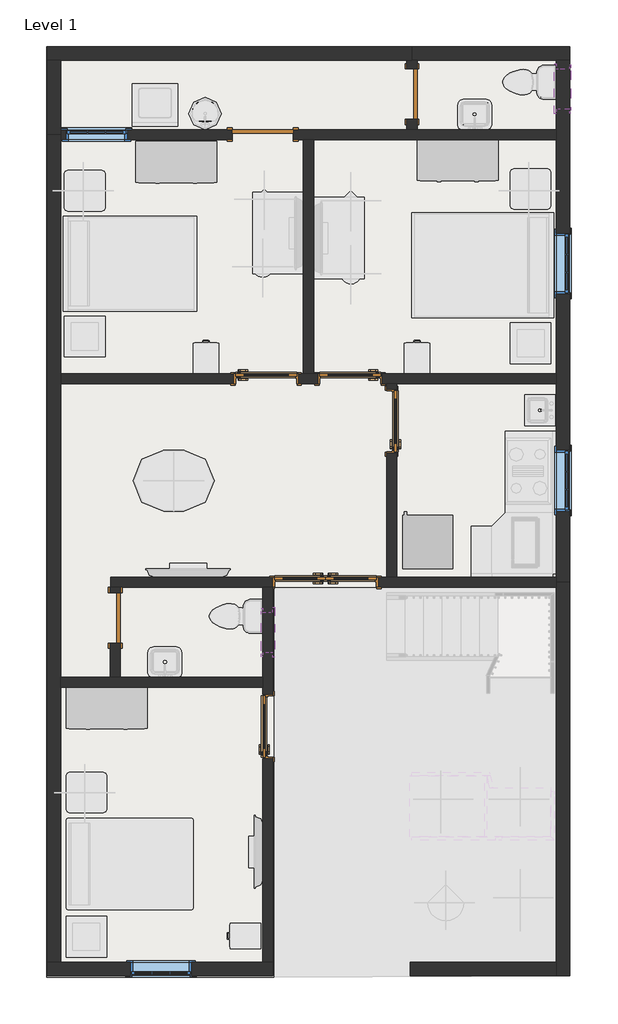
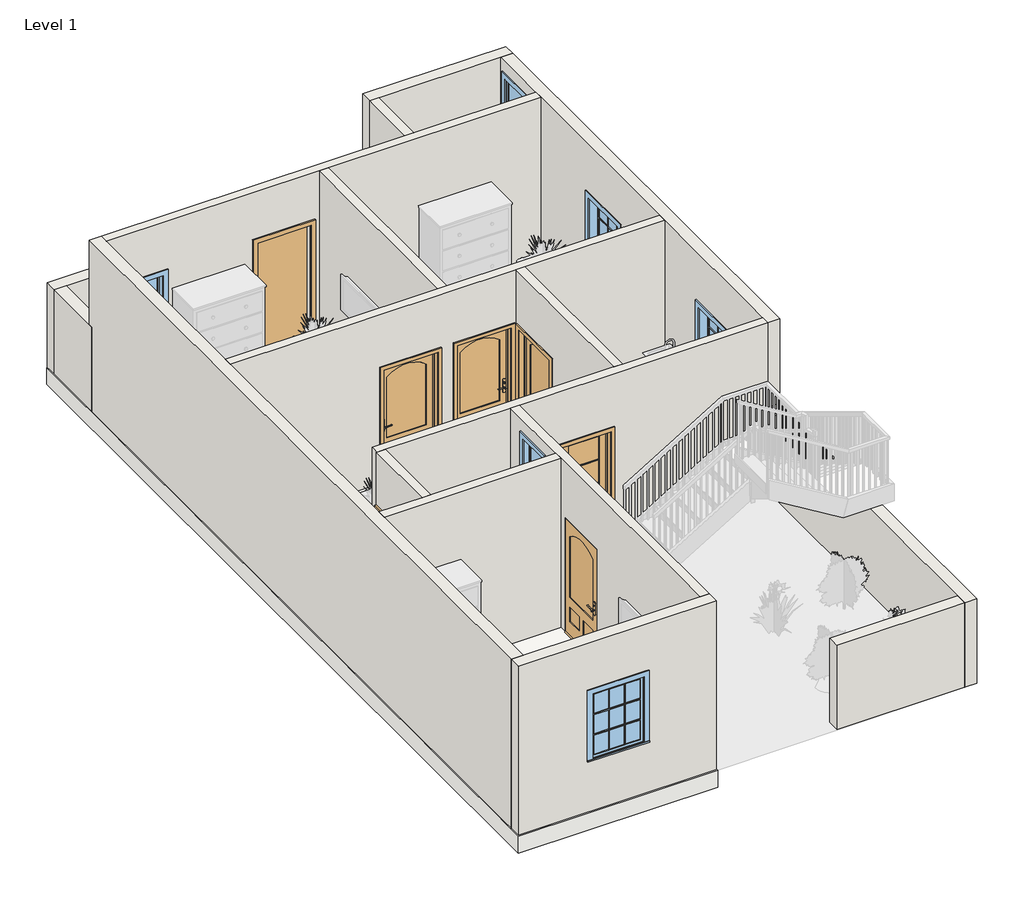
# One storey, part 1 of 4: 17 walls, 8 doors, 6 windows, 1 slab.
"""IFC4 building model written with IfcOpenShell, lengths in millimetres."""

from ifc_helpers import new_model, si_unit, frame, origin, origin_with_axes, place, context, project, spatial, polyline, outline, extrude, faceted_brep, transform, mapped, element, save
from components import door_5d363d20, door_808aeb8e, door_19287a7a, door_94998e6c, door_255cab33, door_16372e1c, window_5c190c7e, window_29c06734, window_e41d21a6, window_3d781103

model = new_model("IFC4")

# Units and contexts
model_context = context("Model", 3, world=origin())
ifc_project = project(units=[si_unit("LENGTHUNIT", "METRE", prefix="MILLI")], contexts=[model_context])

# Site, building, storey
site = spatial("IfcSite", under=ifc_project)
building = spatial("IfcBuilding", under=site)
storey = spatial("IfcBuildingStorey", under=building, Name="Level 1", Elevation=0.0)

# Doors
placement = place(None, origin())
door_shape = door_5d363d20(model_context)
element("IfcDoor", 1, ObjectType="36\" x 80\"", at=placement, inside=storey, context=model_context, shape_type="MappedRepresentation", body=[
    mapped(door_shape, transform((-11035.3118598, 8508.9118529, 0.0), x_axis=(-1.0, 0.0, 0.0), y_axis=(0.0, -1.0, 0.0), z_axis=(0.0, 0.0, 1.0))),
])
door_2_shape = door_808aeb8e(model_context)
element("IfcDoor", 2, ObjectType="36\" x 80\"", at=placement, inside=storey, context=model_context, shape_type="MappedRepresentation", body=[
    mapped(door_2_shape, transform((-9778.0118598, 8508.9118529, 0.0), x_axis=(1.0, 0.0, 0.0), y_axis=(0.0, 1.0, 0.0), z_axis=(0.0, 0.0, 1.0))),
])
element("IfcDoor", 3, ObjectType="36\" x 80\"", at=placement, inside=storey, context=model_context, shape_type="MappedRepresentation", body=[
    mapped(door_2_shape, transform((-9152.5368598, 7870.7368529, 0.0), x_axis=(0.0, -1.0, 0.0), y_axis=(1.0, 0.0, 0.0), z_axis=(0.0, 0.0, 1.0))),
])
door_3_shape = door_19287a7a(model_context)
element("IfcDoor", 4, ObjectType="36\" x 80\"", at=placement, inside=storey, context=model_context, shape_type="MappedRepresentation", body=[
    mapped(door_3_shape, transform((-11013.0868598, 3298.7368529, 0.0), x_axis=(0.0, -1.0, 0.0), y_axis=(1.0, 0.0, 0.0), z_axis=(0.0, 0.0, 1.0))),
])
door_4_shape = door_94998e6c(model_context)
element("IfcDoor", 5, ObjectType="Door-Exterior-Double-Full Glass-Wood_Clad : 60\" x 80\"", at=placement, inside=storey, context=model_context, shape_type="MappedRepresentation", body=[
    mapped(door_4_shape, transform((-10146.3118598, 5460.9118529, 0.0), x_axis=(1.0, 0.0, 0.0), y_axis=(0.0, 1.0, 0.0), z_axis=(0.0, 0.0, 1.0))),
])
door_5_shape = door_255cab33(model_context)
element("IfcDoor", 6, ObjectType="Single-Flush : 30\" x 80\"", at=placement, inside=storey, context=model_context, shape_type="MappedRepresentation", body=[
    mapped(door_5_shape, transform((-8850.9118598, 12772.9368529, 0.0), x_axis=(0.0, 1.0, 0.0), y_axis=(-1.0, 0.0, 0.0), z_axis=(0.0, 0.0, 1.0))),
])
element("IfcDoor", 7, ObjectType="Single-Flush : 30\" x 80\"", at=placement, inside=storey, context=model_context, shape_type="MappedRepresentation", body=[
    mapped(door_5_shape, transform((-13295.9118598, 4924.3368529, 0.0), x_axis=(0.0, 1.0, 0.0), y_axis=(-1.0, 0.0, 0.0), z_axis=(0.0, 0.0, 1.0))),
])
door_6_shape = door_16372e1c(model_context)
element("IfcDoor", 8, ObjectType="Single-Flush : 36\" x 84\"", at=placement, inside=storey, context=model_context, shape_type="MappedRepresentation", body=[
    mapped(door_6_shape, transform((-11086.1118598, 12163.3368529, 0.0), x_axis=(1.0, 0.0, 0.0), y_axis=(0.0, 1.0, 0.0), z_axis=(0.0, 0.0, 1.0))),
])

# Slab
element("IfcSlab", 9, ObjectType="Generic - 12\"", at=placement, inside=storey, context=model_context, shape_type="SweptSolid", body=[
    extrude(outline(polyline([(-6488.7118598, 13484.1368529), (-6488.7118598, 5381.5368529), (-10921.0118598, 5381.5368529), (-10921.0118598, -460.4631471), (-14324.6118598, -460.4631471), (-14324.6118598, 13484.1368529), (-6488.7118598, 13484.1368529)])), frame((0.0, 0.0, -304.8), z_axis=(0.0, 0.0, 1.0), x_axis=(1.0, 0.0, 0.0)), (0.0, 0.0, 1.0), 304.8),
])

# Walls
element("IfcWall", 10, ObjectType="Generic - 5'", at=placement, inside=storey, context=model_context, shape_type="Brep", body=[
    faceted_brep([(-14311.9118598, 13280.9368529, 0.0), (-14108.7118598, 13280.9368529, 0.0), (-8927.1118598, 13280.9368529, 0.0), (-8850.9118598, 13280.9368529, 0.0), (-8850.9118598, 13280.9368529, 1524.0), (-14108.7118598, 13280.9368529, 1524.0), (-14311.9118598, 13280.9368529, 1524.0), (-14311.9118598, 13484.1368529, 0.0), (-14311.9118598, 13484.1368529, 1524.0), (-8850.9118598, 13484.1368529, 1524.0), (-8850.9118598, 13484.1368529, 0.0)], [[[0, 1, 2, 3, 4, 5, 6]], [[7, 8, 9, 10]], [[3, 2, 1, 0, 7, 10]], [[4, 3, 10, 9]], [[6, 5, 4, 9, 8]], [[0, 6, 8, 7]]]),
])
element("IfcWall", 11, ObjectType="Generic - 5'", at=placement, inside=storey, context=model_context, shape_type="Brep", body=[
    faceted_brep([(-6691.9118598, 5457.7368529, 0.0), (-6691.9118598, 5381.5368529, 0.0), (-6691.9118598, -231.8631471, 0.0), (-6691.9118598, -435.0631471, 0.0), (-6691.9118598, -435.0631471, 1524.0), (-6691.9118598, -231.8631471, 1524.0), (-6691.9118598, 5457.7368529, 1524.0), (-6488.7118598, 5457.7368529, 0.0), (-6488.7118598, 5457.7368529, 1524.0), (-6488.7118598, -435.0631471, 1524.0), (-6488.7118598, -435.0631471, 0.0)], [[[0, 1, 2, 3, 4, 5, 6]], [[7, 8, 9, 10]], [[3, 2, 1, 0, 7, 10]], [[6, 5, 4, 9, 8]], [[0, 6, 8, 7]], [[4, 3, 10, 9]]]),
])
element("IfcWall", 12, ObjectType="Generic - 5'", at=placement, inside=storey, context=model_context, shape_type="Brep", body=[
    faceted_brep([(-14108.7118598, 12163.3368529, 0.0), (-14108.7118598, 12239.5368529, 0.0), (-14108.7118598, 13280.9368529, 0.0), (-14108.7118598, 13280.9368529, 1524.0), (-14108.7118598, 12163.3368529, 1524.0), (-14311.9118598, 12163.3368529, 0.0), (-14311.9118598, 12163.3368529, 1524.0), (-14311.9118598, 13280.9368529, 1524.0), (-14311.9118598, 13280.9368529, 0.0)], [[[0, 1, 2, 3, 4]], [[5, 6, 7, 8]], [[2, 1, 0, 5, 8]], [[4, 3, 7, 6]], [[0, 4, 6, 5]], [[3, 2, 8, 7]]]),
])
element("IfcWall", 13, ObjectType="Generic - 5'", at=placement, inside=storey, context=model_context, shape_type="SweptSolid", body=[
    extrude(outline(polyline([(-8876.3118598, -231.8631471), (-6691.9118598, -231.8631471), (-6691.9118598, -435.0631471), (-8876.3118598, -435.0631471), (-8876.3118598, -231.8631471)])), origin_with_axes(), (0.0, 0.0, 1.0), 1524.0),
])
element("IfcWall", 14, ObjectType="Generic - 8\"", at=placement, inside=storey, context=model_context, shape_type="Brep", body=[
    faceted_brep([(-6691.9118598, 13280.9368529, 0.0), (-6691.9118598, 12239.5368529, 0.0), (-6691.9118598, 12087.1368529, 0.0), (-6691.9118598, 8581.9368529, 0.0), (-6691.9118598, 8429.5368529, 0.0), (-6691.9118598, 5533.9368529, 0.0), (-6691.9118598, 5457.7368529, 0.0), (-6691.9118598, 5457.7368529, 1524.0), (-6691.9118598, 5381.5368529, 1524.0), (-6691.9118598, 5381.5368529, 3048.0), (-6691.9118598, 5533.9368529, 3048.0), (-6691.9118598, 8429.5368529, 3048.0), (-6691.9118598, 8581.9368529, 3048.0), (-6691.9118598, 12087.1368529, 3048.0), (-6691.9118598, 12239.5368529, 3048.0), (-6691.9118598, 13280.9368529, 3048.0), (-6691.9118598, 9775.7368529, 2133.6), (-6691.9118598, 9775.7368529, 914.4), (-6691.9118598, 10690.1368529, 914.4), (-6691.9118598, 10690.1368529, 2133.6), (-6691.9118598, 6524.5368529, 2133.6), (-6691.9118598, 6524.5368529, 914.4), (-6691.9118598, 7438.9368529, 914.4), (-6691.9118598, 7438.9368529, 2133.6), (-6691.9118598, 13153.9368529, 2768.6), (-6691.9118598, 12544.3368529, 2768.6), (-6691.9118598, 12544.3368529, 2159.0), (-6691.9118598, 13153.9368529, 2159.0), (-6488.7118598, 13280.9368529, 0.0), (-6488.7118598, 13280.9368529, 3048.0), (-6488.7118598, 5381.5368529, 3048.0), (-6488.7118598, 5381.5368529, 1524.0), (-6488.7118598, 5457.7368529, 1524.0), (-6488.7118598, 5457.7368529, 0.0), (-6488.7118598, 9775.7368529, 2133.6), (-6488.7118598, 10690.1368529, 2133.6), (-6488.7118598, 10690.1368529, 914.4), (-6488.7118598, 9775.7368529, 914.4), (-6488.7118598, 6524.5368529, 2133.6), (-6488.7118598, 7438.9368529, 2133.6), (-6488.7118598, 7438.9368529, 914.4), (-6488.7118598, 6524.5368529, 914.4), (-6488.7118598, 13153.9368529, 2768.6), (-6488.7118598, 13153.9368529, 2159.0), (-6488.7118598, 12544.3368529, 2159.0), (-6488.7118598, 12544.3368529, 2768.6)], [[[0, 1, 2, 3, 4, 5, 6, 7, 8, 9, 10, 11, 12, 13, 14, 15], [16, 17, 18, 19], [20, 21, 22, 23], [24, 25, 26, 27]], [[28, 29, 30, 31, 32, 33], [34, 35, 36, 37], [38, 39, 40, 41], [42, 43, 44, 45]], [[6, 5, 4, 3, 2, 1, 0, 28, 33]], [[0, 15, 29, 28]], [[17, 16, 34, 37]], [[18, 17, 37, 36]], [[19, 18, 36, 35]], [[16, 19, 35, 34]], [[21, 20, 38, 41]], [[22, 21, 41, 40]], [[23, 22, 40, 39]], [[20, 23, 39, 38]], [[43, 42, 24, 27]], [[44, 43, 27, 26]], [[45, 44, 26, 25]], [[42, 45, 25, 24]], [[7, 6, 33, 32]], [[31, 8, 7, 32]], [[9, 8, 31, 30]], [[15, 14, 13, 12, 11, 10, 9, 30, 29]]]),
])
element("IfcWall", 15, ObjectType="Generic - 8\"", at=placement, inside=storey, context=model_context, shape_type="Brep", body=[
    faceted_brep([(-14108.7118598, -231.8631471, 0.0), (-14108.7118598, 3882.9368529, 0.0), (-14108.7118598, 4035.3368529, 0.0), (-14108.7118598, 8429.5368529, 0.0), (-14108.7118598, 8581.9368529, 0.0), (-14108.7118598, 12087.1368529, 0.0), (-14108.7118598, 12163.3368529, 0.0), (-14108.7118598, 12163.3368529, 1524.0), (-14108.7118598, 12239.5368529, 1524.0), (-14108.7118598, 12239.5368529, 3048.0), (-14108.7118598, 12087.1368529, 3048.0), (-14108.7118598, 8581.9368529, 3048.0), (-14108.7118598, 8429.5368529, 3048.0), (-14108.7118598, 4035.3368529, 3048.0), (-14108.7118598, 3882.9368529, 3048.0), (-14108.7118598, -231.8631471, 3048.0), (-14311.9118598, -231.8631471, 0.0), (-14311.9118598, -231.8631471, 3048.0), (-14311.9118598, 12239.5368529, 3048.0), (-14311.9118598, 12239.5368529, 1524.0), (-14311.9118598, 12163.3368529, 1524.0), (-14311.9118598, 12163.3368529, 0.0)], [[[0, 1, 2, 3, 4, 5, 6, 7, 8, 9, 10, 11, 12, 13, 14, 15]], [[16, 17, 18, 19, 20, 21]], [[6, 5, 4, 3, 2, 1, 0, 16, 21]], [[0, 15, 17, 16]], [[7, 6, 21, 20]], [[19, 8, 7, 20]], [[9, 8, 19, 18]], [[15, 14, 13, 12, 11, 10, 9, 18, 17]]]),
])
element("IfcWall", 16, ObjectType="Generic - 8\"", at=placement, inside=storey, context=model_context, shape_type="Brep", body=[
    faceted_brep([(-10933.7118598, -231.8631471, 0.0), (-11086.1118598, -231.8631471, 0.0), (-14108.7118598, -231.8631471, 0.0), (-14311.9118598, -231.8631471, 0.0), (-14311.9118598, -231.8631471, 3048.0), (-14108.7118598, -231.8631471, 3048.0), (-11086.1118598, -231.8631471, 3048.0), (-10933.7118598, -231.8631471, 3048.0), (-13067.3118598, -231.8631471, 2133.6), (-13067.3118598, -231.8631471, 914.4), (-12152.9118598, -231.8631471, 914.4), (-12152.9118598, -231.8631471, 2133.6), (-10933.7118598, -435.0631471, 0.0), (-10933.7118598, -435.0631471, 3048.0), (-14311.9118598, -435.0631471, 3048.0), (-14311.9118598, -435.0631471, 0.0), (-13067.3118598, -435.0631471, 2133.6), (-12152.9118598, -435.0631471, 2133.6), (-12152.9118598, -435.0631471, 914.4), (-13067.3118598, -435.0631471, 914.4)], [[[0, 1, 2, 3, 4, 5, 6, 7], [8, 9, 10, 11]], [[12, 13, 14, 15], [16, 17, 18, 19]], [[3, 2, 1, 0, 12, 15]], [[4, 3, 15, 14]], [[9, 8, 16, 19]], [[10, 9, 19, 18]], [[11, 10, 18, 17]], [[8, 11, 17, 16]], [[0, 7, 13, 12]], [[7, 6, 5, 4, 14, 13]]]),
])
element("IfcWall", 17, ObjectType="Generic - 8\"", at=placement, inside=storey, context=model_context, shape_type="Brep", body=[
    faceted_brep([(-8850.9118598, 13280.9368529, 0.0), (-8774.7118598, 13280.9368529, 0.0), (-6691.9118598, 13280.9368529, 0.0), (-6488.7118598, 13280.9368529, 0.0), (-6488.7118598, 13280.9368529, 3048.0), (-6691.9118598, 13280.9368529, 3048.0), (-8774.7118598, 13280.9368529, 3048.0), (-8927.1118598, 13280.9368529, 3048.0), (-8927.1118598, 13280.9368529, 1524.0), (-8850.9118598, 13280.9368529, 1524.0), (-8850.9118598, 13484.1368529, 0.0), (-8850.9118598, 13484.1368529, 1524.0), (-8927.1118598, 13484.1368529, 1524.0), (-8927.1118598, 13484.1368529, 3048.0), (-6488.7118598, 13484.1368529, 3048.0), (-6488.7118598, 13484.1368529, 0.0)], [[[0, 1, 2, 3, 4, 5, 6, 7, 8, 9]], [[10, 11, 12, 13, 14, 15]], [[3, 2, 1, 0, 10, 15]], [[4, 3, 15, 14]], [[0, 9, 11, 10]], [[8, 12, 11, 9]], [[8, 7, 13, 12]], [[7, 6, 5, 4, 14, 13]]]),
])
element("IfcWall", 18, ObjectType="INNER 6\"", at=placement, inside=storey, context=model_context, shape_type="Brep", body=[
    faceted_brep([(-10628.9118598, 12087.1368529, 2133.6), (-10628.9118598, 12087.1368529, 0.0), (-10476.5118598, 12087.1368529, 0.0), (-10324.1118598, 12087.1368529, 0.0), (-6691.9118598, 12087.1368529, 0.0), (-6691.9118598, 12087.1368529, 3048.0), (-10324.1118598, 12087.1368529, 3048.0), (-10476.5118598, 12087.1368529, 3048.0), (-14108.7118598, 12087.1368529, 3048.0), (-14108.7118598, 12087.1368529, 0.0), (-11543.3118598, 12087.1368529, 0.0), (-11543.3118598, 12087.1368529, 2133.6), (-13118.1118598, 12087.1368529, 2133.6), (-13118.1118598, 12087.1368529, 914.4), (-14032.5118598, 12087.1368529, 914.4), (-14032.5118598, 12087.1368529, 2133.6), (-6691.9118598, 12239.5368529, 0.0), (-8774.7118598, 12239.5368529, 0.0), (-8927.1118598, 12239.5368529, 0.0), (-10628.9118598, 12239.5368529, 0.0), (-10628.9118598, 12239.5368529, 2133.6), (-11543.3118598, 12239.5368529, 2133.6), (-11543.3118598, 12239.5368529, 0.0), (-14108.7118598, 12239.5368529, 0.0), (-14108.7118598, 12239.5368529, 1524.0), (-14108.7118598, 12239.5368529, 3048.0), (-8927.1118598, 12239.5368529, 3048.0), (-8774.7118598, 12239.5368529, 3048.0), (-6691.9118598, 12239.5368529, 3048.0), (-13118.1118598, 12239.5368529, 2133.6), (-14032.5118598, 12239.5368529, 2133.6), (-14032.5118598, 12239.5368529, 914.4), (-13118.1118598, 12239.5368529, 914.4), (-14108.7118598, 12163.3368529, 0.0)], [[[0, 1, 2, 3, 4, 5, 6, 7, 8, 9, 10, 11], [12, 13, 14, 15]], [[16, 17, 18, 19, 20, 21, 22, 23, 24, 25, 26, 27, 28], [29, 30, 31, 32]], [[10, 9, 33, 23, 22]], [[4, 3, 2, 1, 19, 18, 17, 16]], [[5, 4, 16, 28]], [[20, 19, 1, 0]], [[21, 20, 0, 11]], [[22, 21, 11, 10]], [[13, 12, 29, 32]], [[14, 13, 32, 31]], [[15, 14, 31, 30]], [[12, 15, 30, 29]], [[8, 25, 24, 23, 33, 9]], [[8, 7, 6, 5, 28, 27, 26, 25]]]),
])
element("IfcWall", 19, ObjectType="INNER 6\"", at=placement, inside=storey, context=model_context, shape_type="Brep", body=[
    faceted_brep([(-8927.1118598, 13280.9368529, 0.0), (-8927.1118598, 13153.9368529, 0.0), (-8927.1118598, 13153.9368529, 2032.0), (-8927.1118598, 12391.9368529, 2032.0), (-8927.1118598, 12391.9368529, 0.0), (-8927.1118598, 12239.5368529, 0.0), (-8927.1118598, 12239.5368529, 3048.0), (-8927.1118598, 13280.9368529, 3048.0), (-8927.1118598, 13280.9368529, 1524.0), (-8774.7118598, 13153.9368529, 2032.0), (-8774.7118598, 13153.9368529, 0.0), (-8774.7118598, 13280.9368529, 0.0), (-8774.7118598, 13280.9368529, 3048.0), (-8774.7118598, 12239.5368529, 3048.0), (-8774.7118598, 12239.5368529, 0.0), (-8774.7118598, 12391.9368529, 0.0), (-8774.7118598, 12391.9368529, 2032.0), (-8850.9118598, 13280.9368529, 0.0)], [[[0, 1, 2, 3, 4, 5, 6, 7, 8]], [[9, 10, 11, 12, 13, 14, 15, 16]], [[15, 14, 5, 4]], [[11, 10, 1, 0, 17]], [[6, 5, 14, 13]], [[2, 1, 10, 9]], [[3, 2, 9, 16]], [[4, 3, 16, 15]], [[7, 12, 11, 17, 0, 8]], [[7, 6, 13, 12]]]),
])
element("IfcWall", 20, ObjectType="INNER 6\"", at=placement, inside=storey, context=model_context, shape_type="Brep", body=[
    faceted_brep([(-6691.9118598, 8429.5368529, 0.0), (-6691.9118598, 8429.5368529, 3048.0), (-9079.5118598, 8429.5368529, 3048.0), (-9231.9118598, 8429.5368529, 3048.0), (-14108.7118598, 8429.5368529, 3048.0), (-14108.7118598, 8429.5368529, 0.0), (-11517.9118598, 8429.5368529, 0.0), (-11517.9118598, 8429.5368529, 2057.4), (-10552.7118598, 8429.5368529, 2057.4), (-10552.7118598, 8429.5368529, 0.0), (-10260.6118598, 8429.5368529, 0.0), (-10260.6118598, 8429.5368529, 2057.4), (-9295.4118598, 8429.5368529, 2057.4), (-9295.4118598, 8429.5368529, 0.0), (-9231.9118598, 8429.5368529, 0.0), (-9079.5118598, 8429.5368529, 0.0), (-6691.9118598, 8581.9368529, 3048.0), (-6691.9118598, 8581.9368529, 0.0), (-9295.4118598, 8581.9368529, 0.0), (-9295.4118598, 8581.9368529, 2057.4), (-10260.6118598, 8581.9368529, 2057.4), (-10260.6118598, 8581.9368529, 0.0), (-10324.1118598, 8581.9368529, 0.0), (-10476.5118598, 8581.9368529, 0.0), (-10552.7118598, 8581.9368529, 0.0), (-10552.7118598, 8581.9368529, 2057.4), (-11517.9118598, 8581.9368529, 2057.4), (-11517.9118598, 8581.9368529, 0.0), (-14108.7118598, 8581.9368529, 0.0), (-14108.7118598, 8581.9368529, 3048.0), (-10476.5118598, 8581.9368529, 3048.0), (-10324.1118598, 8581.9368529, 3048.0)], [[[0, 1, 2, 3, 4, 5, 6, 7, 8, 9, 10, 11, 12, 13, 14, 15]], [[16, 17, 18, 19, 20, 21, 22, 23, 24, 25, 26, 27, 28, 29, 30, 31]], [[5, 28, 27, 6]], [[17, 0, 15, 14, 13, 18]], [[9, 24, 23, 22, 21, 10]], [[1, 0, 17, 16]], [[5, 4, 29, 28]], [[26, 7, 6, 27]], [[7, 26, 25, 8]], [[8, 25, 24, 9]], [[12, 19, 18, 13]], [[19, 12, 11, 20]], [[20, 11, 10, 21]], [[4, 3, 2, 1, 16, 31, 30, 29]]]),
])
element("IfcWall", 21, ObjectType="INNER 6\"", at=placement, inside=storey, context=model_context, shape_type="SweptSolid", body=[
    extrude(outline(polyline([(-10476.5118598, 8581.9368529), (-10476.5118598, 12087.1368529), (-10324.1118598, 12087.1368529), (-10324.1118598, 8581.9368529), (-10476.5118598, 8581.9368529)])), origin_with_axes(), (0.0, 0.0, 1.0), 3048.0),
])
element("IfcWall", 22, ObjectType="INNER 6\"", at=placement, inside=storey, context=model_context, shape_type="SweptSolid", body=[
    extrude(outline(polyline([(8429.5368529, 3048.0), (8429.5368529, 0.0), (8353.3368529, 0.0), (8353.3368529, 2057.4), (7388.1368529, 2057.4), (7388.1368529, 0.0), (5533.9368529, 0.0), (5533.9368529, 3048.0), (8429.5368529, 3048.0)])), frame((-9231.9118598, 0.0, 0.0), z_axis=(1.0, 0.0, 0.0), x_axis=(0.0, 1.0, 0.0)), (0.0, 0.0, 1.0), 152.4),
])
element("IfcWall", 23, ObjectType="INNER 6\"", at=placement, inside=storey, context=model_context, shape_type="Brep", body=[
    faceted_brep([(-14108.7118598, 3882.9368529, 0.0), (-11086.1118598, 3882.9368529, 0.0), (-11086.1118598, 3882.9368529, 3048.0), (-14108.7118598, 3882.9368529, 3048.0), (-14108.7118598, 4035.3368529, 0.0), (-14108.7118598, 4035.3368529, 3048.0), (-13372.1118598, 4035.3368529, 3048.0), (-13219.7118598, 4035.3368529, 3048.0), (-11086.1118598, 4035.3368529, 3048.0), (-11086.1118598, 4035.3368529, 0.0), (-13219.7118598, 4035.3368529, 0.0), (-13372.1118598, 4035.3368529, 0.0)], [[[0, 1, 2, 3]], [[4, 5, 6, 7, 8, 9, 10, 11]], [[1, 0, 4, 11, 10, 9]], [[0, 3, 5, 4]], [[2, 1, 9, 8]], [[3, 2, 8, 7, 6, 5]]]),
])
element("IfcWall", 24, ObjectType="INNER 6\"", at=placement, inside=storey, context=model_context, shape_type="Brep", body=[
    faceted_brep([(-13219.7118598, 5305.3368529, 2032.0), (-13219.7118598, 5305.3368529, 0.0), (-13219.7118598, 5381.5368529, 0.0), (-13219.7118598, 5381.5368529, 3048.0), (-13219.7118598, 4035.3368529, 3048.0), (-13219.7118598, 4035.3368529, 0.0), (-13219.7118598, 4543.3368529, 0.0), (-13219.7118598, 4543.3368529, 2032.0), (-13372.1118598, 5381.5368529, 0.0), (-13372.1118598, 5305.3368529, 0.0), (-13372.1118598, 5305.3368529, 2032.0), (-13372.1118598, 4543.3368529, 2032.0), (-13372.1118598, 4543.3368529, 0.0), (-13372.1118598, 4035.3368529, 0.0), (-13372.1118598, 4035.3368529, 3048.0), (-13372.1118598, 5381.5368529, 3048.0), (-13359.4118598, 5381.5368529, 0.0), (-13359.4118598, 5381.5368529, 3048.0)], [[[0, 1, 2, 3, 4, 5, 6, 7]], [[8, 9, 10, 11, 12, 13, 14, 15]], [[6, 5, 13, 12]], [[2, 1, 9, 8, 16]], [[3, 2, 16, 8, 15, 17]], [[5, 4, 14, 13]], [[10, 9, 1, 0]], [[11, 10, 0, 7]], [[12, 11, 7, 6]], [[4, 3, 17, 15, 14]]]),
])
element("IfcWall", 25, ObjectType="INNER 6\"", at=placement, inside=storey, context=model_context, shape_type="Brep", body=[
    faceted_brep([(-10933.7118598, 5381.5368529, 0.0), (-10933.7118598, 5381.5368529, 2057.4), (-10933.7118598, 5381.5368529, 3048.0), (-10933.7118598, -231.8631471, 3048.0), (-10933.7118598, -231.8631471, 0.0), (-10933.7118598, 2816.1368529, 0.0), (-10933.7118598, 2816.1368529, 2057.4), (-10933.7118598, 3781.3368529, 2057.4), (-10933.7118598, 3781.3368529, 0.0), (-10933.7118598, 4403.6368529, 2768.6), (-10933.7118598, 5013.2368529, 2768.6), (-10933.7118598, 5013.2368529, 2159.0), (-10933.7118598, 4403.6368529, 2159.0), (-11086.1118598, 5381.5368529, 3048.0), (-11086.1118598, 5381.5368529, 0.0), (-11086.1118598, 4035.3368529, 0.0), (-11086.1118598, 3882.9368529, 0.0), (-11086.1118598, 3781.3368529, 0.0), (-11086.1118598, 3781.3368529, 2057.4), (-11086.1118598, 2816.1368529, 2057.4), (-11086.1118598, 2816.1368529, 0.0), (-11086.1118598, -231.8631471, 0.0), (-11086.1118598, -231.8631471, 3048.0), (-11086.1118598, 3882.9368529, 3048.0), (-11086.1118598, 4035.3368529, 3048.0), (-11086.1118598, 4403.6368529, 2768.6), (-11086.1118598, 4403.6368529, 2159.0), (-11086.1118598, 5013.2368529, 2159.0), (-11086.1118598, 5013.2368529, 2768.6)], [[[0, 1, 2, 3, 4, 5, 6, 7, 8], [9, 10, 11, 12]], [[13, 14, 15, 16, 17, 18, 19, 20, 21, 22, 23, 24], [25, 26, 27, 28]], [[14, 0, 8, 17, 16, 15]], [[4, 21, 20, 5]], [[2, 1, 0, 14, 13]], [[4, 3, 22, 21]], [[19, 6, 5, 20]], [[6, 19, 18, 7]], [[7, 18, 17, 8]], [[26, 25, 9, 12]], [[27, 26, 12, 11]], [[28, 27, 11, 10]], [[25, 28, 10, 9]], [[3, 2, 13, 24, 23, 22]]]),
])
element("IfcWall", 26, ObjectType="INNER 6\"", at=placement, inside=storey, context=model_context, shape_type="Brep", body=[
    faceted_brep([(-13359.4118598, 5381.5368529, 3048.0), (-13359.4118598, 5381.5368529, 0.0), (-13219.7118598, 5381.5368529, 0.0), (-11086.1118598, 5381.5368529, 0.0), (-10933.7118598, 5381.5368529, 0.0), (-10933.7118598, 5381.5368529, 2057.4), (-9358.9118598, 5381.5368529, 2057.4), (-9358.9118598, 5381.5368529, 0.0), (-6691.9118598, 5381.5368529, 0.0), (-6691.9118598, 5381.5368529, 1524.0), (-6691.9118598, 5381.5368529, 3048.0), (-10933.7118598, 5381.5368529, 3048.0), (-11086.1118598, 5381.5368529, 3048.0), (-13219.7118598, 5381.5368529, 3048.0), (-13359.4118598, 5533.9368529, 0.0), (-13359.4118598, 5533.9368529, 3048.0), (-9231.9118598, 5533.9368529, 3048.0), (-9079.5118598, 5533.9368529, 3048.0), (-6691.9118598, 5533.9368529, 3048.0), (-6691.9118598, 5533.9368529, 0.0), (-9079.5118598, 5533.9368529, 0.0), (-9231.9118598, 5533.9368529, 0.0), (-9358.9118598, 5533.9368529, 0.0), (-9358.9118598, 5533.9368529, 2057.4), (-10933.7118598, 5533.9368529, 2057.4), (-10933.7118598, 5533.9368529, 0.0), (-6691.9118598, 5457.7368529, 0.0)], [[[0, 1, 2, 3, 4, 5, 6, 7, 8, 9, 10, 11, 12, 13]], [[14, 15, 16, 17, 18, 19, 20, 21, 22, 23, 24, 25]], [[1, 14, 25, 4, 3, 2]], [[19, 26, 8, 7, 22, 21, 20]], [[1, 0, 15, 14]], [[6, 23, 22, 7]], [[23, 6, 5, 24]], [[24, 5, 4, 25]], [[8, 26, 19, 18, 10, 9]], [[0, 13, 12, 11, 10, 18, 17, 16, 15]]]),
])

# Windows
window_shape = window_5c190c7e(model_context)
element("IfcWindow", 27, ObjectType="Casement 3x3 with Trim : 36\" x 48\"", at=placement, inside=storey, context=model_context, shape_type="MappedRepresentation", body=[
    mapped(window_shape, transform((-13575.3118598, 12163.3368529, 0.0), x_axis=(1.0, 0.0, 0.0), y_axis=(0.0, 1.0, 0.0), z_axis=(0.0, 0.0, 1.0))),
])
window_2_shape = window_29c06734(model_context)
element("IfcWindow", 28, ObjectType="Casement 3x3 with Trim : 36\" x 48\"", at=placement, inside=storey, context=model_context, shape_type="MappedRepresentation", body=[
    mapped(window_2_shape, transform((-6590.3118598, 10232.9368529, 0.0), x_axis=(0.0, -1.0, 0.0), y_axis=(1.0, 0.0, 0.0), z_axis=(0.0, 0.0, 1.0))),
])
element("IfcWindow", 29, ObjectType="Casement 3x3 with Trim : 36\" x 48\"", at=placement, inside=storey, context=model_context, shape_type="MappedRepresentation", body=[
    mapped(window_2_shape, transform((-6590.3118598, 6981.7368529, 0.0), x_axis=(0.0, -1.0, 0.0), y_axis=(1.0, 0.0, 0.0), z_axis=(0.0, 0.0, 1.0))),
])
element("IfcWindow", 30, ObjectType="Casement 3x3 with Trim : 36\" x 48\"", at=placement, inside=storey, context=model_context, shape_type="MappedRepresentation", body=[
    mapped(window_2_shape, transform((-12610.1118598, -333.4631471, 0.0), x_axis=(-1.0, 0.0, 0.0), y_axis=(0.0, -1.0, 0.0), z_axis=(0.0, 0.0, 1.0))),
])
window_3_shape = window_e41d21a6(model_context)
element("IfcWindow", 31, ObjectType="Transom with Trim : 24\" x 24\"", at=placement, inside=storey, context=model_context, shape_type="MappedRepresentation", body=[
    mapped(window_3_shape, transform((-6590.3118598, 12887.2368529, 0.0), x_axis=(0.0, 1.0, 0.0), y_axis=(-1.0, 0.0, 0.0), z_axis=(0.0, 0.0, 1.0))),
])
window_4_shape = window_3d781103(model_context)
element("IfcWindow", 32, ObjectType="Transom with Trim : 24\" x 24\"", at=placement, inside=storey, context=model_context, shape_type="MappedRepresentation", body=[
    mapped(window_4_shape, transform((-11009.9118598, 4670.3368529, 0.0), x_axis=(0.0, -1.0, 0.0), y_axis=(1.0, 0.0, 0.0), z_axis=(0.0, 0.0, 1.0))),
])

save(model, "model.ifc")

# Revit data of these elements
# Type "36\" x 80\""
#   Type Mark = "8"
#   Assembly Code = "B2030100"
#   Analytic Construction = "French door, wood frame with single glass"
#   Threshold Offset [instance default] = 0' - 0 1/2"
#   Thickness = 0' - 1 3/8"
#   Thermal Resistance (R) = 1.0696 (h·ft²·°F)/BTU
#   Swing Angle [instance default] = 90.00°
#   Stiles = 0' - 4 3/4"
#   Rough Width = 3' - 2"
#   Rough Height = 6' - 9"
#   Radius = 1' - 8.05625"
#   Lock Rail = 0' - 7 1/8"
#   Height = 6' - 8"
#   Width = 3' - 0"
#   Heat Transfer Coefficient (U) = 0.9350 BTU/(h·ft²·°F)
#   Door Offset [instance default] = 0' - 0"
#   Bottom Rail = 0' - 9 1/2"
#   Threshold [instance default] = yes
#   Function = 1
#   Exterior Trim [instance default] = yes
#   Trim Material = Cherry
#   Threshold Material = Cherry
#   Panel Material = Cherry
#   Glazing = Glass
#   Frame Material = Cherry
#   Door Handle Material = Aluminum
#   Visual Light Transmittance = 0
#   Solar Heat Gain Coefficient = 0
#   Wall Closure = (empty or 0)
#   Construction Type = (empty or 0)
# Type "Door-Exterior-Double-Full Glass-Wood_Clad : 60\" x 80\""
#   Type Mark = "9"
#   Assembly Code = "B2030100"
#   Analytic Construction = "French door, wood frame with double glass"
#   Top Rail = 0' - 4 11/16"
#   Threshold Offset [instance default] = 0' - 0 1/2"
#   Thickness = 0' - 1 3/8"
#   Thermal Resistance (R) = 1.9158 (h·ft²·°F)/BTU
#   Swing Angle [instance default] = 90.00°
#   Stiles = 0' - 4 3/4"
#   Rough Width = 5' - 2"
#   Rough Height = 6' - 9"
#   Panel Width = 2' - 6"
#   Door Offset [instance default] = 0' - 0"
#   Height = 6' - 8"
#   Width = 5' - 0"
#   Heat Transfer Coefficient (U) = 0.5220 BTU/(h·ft²·°F)
#   Bottom Rail = 0' - 9 1/8"
#   Exterior Trim [instance default] = yes
#   Threshold [instance default] = yes
#   Show Grill [instance default] = yes
#   Function = 1
#   Trim Material = Cherry
#   Threshold Material = Cherry
#   Panel Material = Cherry
#   Glazing = Glass
#   Frame Material = Cherry
#   Door Handle Material = Aluminum
#   Visual Light Transmittance = 0
#   Solar Heat Gain Coefficient = 0
#   Wall Closure = (empty or 0)
#   Construction Type = (empty or 0)
# Type "Single-Flush : 30\" x 80\""
#   Type Mark = "5"
#   Construction Type Id = "MDOOR"
#   Assembly Code = "C1020"
#   Analytic Construction = "Metal"
#   Thickness = 0' - 2"
#   Heat Transfer Coefficient (U) = 0.651978 BTU/(h·ft²·°F)
#   Height = 6' - 8"
#   Trim Projection Ext = 0' - 1"
#   Trim Projection Int = 0' - 1"
#   Trim Width = 0' - 3"
#   Width = 2' - 6"
#   Define Thermal Properties by = 1
#   Door Material = Door - Panel
#   Frame Material = Door - Frame
#   Visual Light Transmittance = 0
#   Solar Heat Gain Coefficient = 0
#   Function = (empty or 0)
#   Wall Closure = (empty or 0)
# Type "Single-Flush : 36\" x 84\""
#   Type Mark = "1"
#   Construction Type Id = "MDOOR"
#   Assembly Code = "C1020"
#   Analytic Construction = "Metal"
#   Thickness = 0' - 2"
#   Heat Transfer Coefficient (U) = 0.651978 BTU/(h·ft²·°F)
#   Height = 7' - 0"
#   Trim Projection Ext = 0' - 1"
#   Trim Projection Int = 0' - 1"
#   Trim Width = 0' - 3"
#   Width = 3' - 0"
#   Define Thermal Properties by = 1
#   Door Material = Door - Panel
#   Frame Material = Door - Frame
#   Visual Light Transmittance = 0
#   Solar Heat Gain Coefficient = 0
#   Function = (empty or 0)
#   Wall Closure = (empty or 0)
# Type "Generic - 12\""
#   Assembly Code = "B1010"
#   Function = 0
#   Layers, outside or top first: 1' - 0" no material (function 1)
# Type "Generic - 5'"
#   Assembly Code = "B2010"
#   Layers, outside or top first: 0' - 8" "Birch" (function 1)
# Type "Generic - 8\""
#   Assembly Code = "B2010"
#   Layers, outside or top first: 0' - 8" "Brick, Common" (function 1)
# Type "INNER 6\""
#   Assembly Code = "B2010"
#   Layers, outside or top first: 0' - 6" "Brick, Common" (function 1)
# Type "Casement 3x3 with Trim : 36\" x 48\""
#   Type Mark = "10"
#   Construction Type Id = "GSP4R"
#   Assembly Code = "B2020100"
#   Analytic Construction = "1/8 in Pilkington single glazing"
#   Visual Light Transmittance = 0.9
#   Solar Heat Gain Coefficient = 0.78
#   Heat Transfer Coefficient (U) = 0.6496 BTU/(h·ft²·°F)
#   Height = 4' - 0"
#   Default Sill Height = 3' - 0"
#   Trim Projection - Ext. = 0' - 0 1/2"
#   Trim Projection - Int. = 0' - 0 3/4"
#   Trim Width - Exterior = 0' - 3 1/2"
#   Trim Width - Interior = 0' - 3 1/2"
#   Width = 3' - 0"
#   Window Inset = 0' - 0 3/4"
#   Define Thermal Properties by = 1
#   Glass Pane Material = Glass
#   Sash Material = Sash
#   Trim Exterior Material = Trim
#   Trim Interior Material = Trim
#   Wall Closure = (empty or 0)
# Type "Transom with Trim : 24\" x 24\""
#   Type Mark = "13"
#   Construction Type Id = "GSP4R"
#   Assembly Code = "B2020100"
#   Analytic Construction = "1/8 in Pilkington single glazing"
#   Visual Light Transmittance = 0.9
#   Solar Heat Gain Coefficient = 0.78
#   Heat Transfer Coefficient (U) = 0.6496 BTU/(h·ft²·°F)
#   Height = 2' - 0"
#   Default Sill Height = 7' - 1"
#   Trim Projection - Ext. = 0' - 0 1/2"
#   Trim Projection - Int. = 0' - 0 3/4"
#   Trim Width - Exterior = 0' - 3 1/2"
#   Trim Width - Interior = 0' - 3 1/2"
#   Width = 2' - 0"
#   Window Inset = 0' - 0 3/4"
#   Define Thermal Properties by = 1
#   Glass Pane Material = Glass
#   Sash Material = Sash
#   Trim Exterior Material = Trim
#   Trim Interior Material = Trim
#   Wall Closure = (empty or 0)
# Elements 1, 2, 3 (IfcDoor, "36\" x 80\"")
#   Threshold Offset = 0' - 0 1/2"
#   Swing Angle = 90.00°
#   Door Offset = 0' - 0"
#   Threshold = yes
#   Exterior Trim = yes
#   Phase Created = New Construction
#   Materials on its faces: "Cherry", "Aluminum", "Glass"
# Element 4 (IfcDoor, "36\" x 80\"")
#   Threshold Offset = 0' - 0 1/2"
#   Swing Angle = 90.00°
#   Door Offset = 0' - 0.16252"
#   Threshold = yes
#   Exterior Trim = no
#   Phase Created = New Construction
#   Materials on its faces: "Cherry", "Aluminum", "Glass"
# Element 5 (IfcDoor, "Door-Exterior-Double-Full Glass-Wood_Clad : 60\" x 80\"")
#   Threshold Offset = 0' - 0 1/2"
#   Swing Angle = 90.00°
#   Door Offset = 0' - 0"
#   Threshold = yes
#   Show Grill = yes
#   Exterior Trim = yes
#   Phase Created = New Construction
#   Materials on its faces: "Cherry", "Aluminum", "Glass"
# Elements 6, 7 (IfcDoor, "Single-Flush : 30\" x 80\"")
#   Phase Created = New Construction
#   Materials on its faces: "Door - Frame", "Door - Panel"
# Element 8 (IfcDoor, "Single-Flush : 36\" x 84\"")
#   Phase Created = New Construction
#   Materials on its faces: "Door - Frame", "Door - Panel"
# Element 9 (IfcSlab, "Generic - 12\"")
#   Height Offset From Level = 0' - 0"
#   Phase Created = New Construction
#   Materials on its faces: "Default Floor"
# Elements 10, 11, 12, 13 (IfcWall, "Generic - 5'")
#   Top Offset = 0' - 0"
#   Base Offset = 0' - 0"
#   Unconnected Height = 5' - 0"
#   wall height = 5' - 0"
#   Phase Created = New Construction
#   Base Constraint = Level 1
#   Materials on its faces: "Birch"
# Elements 14, 15, 16, 17 (IfcWall, "Generic - 8\"")
#   Top Offset = 0' - 0"
#   Base Offset = 0' - 0"
#   Unconnected Height = 10' - 0"
#   wall height = 10' - 0"
#   Phase Created = New Construction
#   Base Constraint = Level 1
#   Materials on its faces: "Brick, Common"
# Elements 18, 19, 20, 21, 22, 23, 24, 25, 26 (IfcWall, "INNER 6\"")
#   Top Offset = 0' - 0"
#   Base Offset = 0' - 0"
#   Unconnected Height = 10' - 0"
#   wall height = 10' - 0"
#   Phase Created = New Construction
#   Base Constraint = Level 1
#   Materials on its faces: "Brick, Common"
# Element 27 (IfcWindow, "Casement 3x3 with Trim : 36\" x 48\"")
#   Mark = "1"
#   Phase Created = New Construction
#   Materials on its faces: "Sash", "Glass", "Trim"
# Element 28 (IfcWindow, "Casement 3x3 with Trim : 36\" x 48\"")
#   Mark = "2"
#   Phase Created = New Construction
#   Materials on its faces: "Sash", "Glass", "Trim"
# Element 29 (IfcWindow, "Casement 3x3 with Trim : 36\" x 48\"")
#   Mark = "3"
#   Phase Created = New Construction
#   Materials on its faces: "Sash", "Glass", "Trim"
# Element 30 (IfcWindow, "Casement 3x3 with Trim : 36\" x 48\"")
#   Mark = "4"
#   Phase Created = New Construction
#   Materials on its faces: "Sash", "Glass", "Trim"
# Element 31 (IfcWindow, "Transom with Trim : 24\" x 24\"")
#   Mark = "5"
#   Phase Created = New Construction
#   Materials on its faces: "Sash", "Trim", "Glass"
# Element 32 (IfcWindow, "Transom with Trim : 24\" x 24\"")
#   Mark = "6"
#   Phase Created = New Construction
#   Materials on its faces: "Sash", "Trim", "Glass"
# Materials
#   "Cherry": class "Wood", colour RGB 226 177 128, transparency 0, Description = "Prunus Serotina", Cost = 0
#   "Glass": class "Glass", colour RGB 0 128 192, transparency 0.75, Description = "Soda Lime Glass", Cost = 0
#   "Aluminum": class "Metal", colour RGB 247 247 247, transparency 0, Description = "Aluminum 6061", Cost = 0
#   "Door - Panel": class "Wood", colour RGB 210 159 95, transparency 0
#   "Door - Frame": colour RGB 118 70 51, transparency 0
#   "Birch": class "Wood", colour RGB 224 178 126, transparency 0, Description = "Betula Alleghaniensis", Cost = 0
#   "Brick, Common": class "Masonry", colour RGB 170 98 104, transparency 0, Description = "Common brick", Cost = 0
#   "Sash": class "Wood", colour RGB 224 178 126, transparency 0
#   "Trim": class "Wood", colour RGB 224 178 126, transparency 0
#   "Default Floor": colour RGB 128 128 128, transparency 0
# Room at (-11804.479, 12614.21) mm, phase "New Construction", upper level "Level 1", upper offset 10' - 0", lower offset 0' - 0"
#   Number = "1"
# Room at (-12107.024, 10517.256) mm, phase "New Construction", upper level "Level 1", upper offset 10' - 0", lower offset 0' - 0"
#   Number = "2"
#   Name = "BEDROOM-1"
# Room at (-7830.797, 6775.662) mm, phase "New Construction", upper level "Level 1", upper offset 10' - 0", lower offset 0' - 0"
#   Number = "8"
#   Name = "KITCHEN"
# Room at (-7598.095, 12538.01) mm, phase "New Construction", upper level "Level 1", upper offset 10' - 0", lower offset 0' - 0"
#   Number = "3"
# Room at (-8426.945, 10517.256) mm, phase "New Construction", upper level "Level 1", upper offset 10' - 0", lower offset 0' - 0"
#   Number = "4"
#   Name = "BEDROOM-2"
# Room at (-11617.166, 6775.662) mm, phase "New Construction", upper level "Level 1", upper offset 10' - 0", lower offset 0' - 0"
#   Number = "5"
#   Name = "LIVING/DINING"
# Room at (-12131.567, 4539.569) mm, phase "New Construction", upper level "Level 1", upper offset 10' - 0", lower offset 0' - 0"
#   Number = "6"
#   Name = "BATH"
# Room at (-12686.153, 1557.983) mm, phase "New Construction", upper level "Level 1", upper offset 10' - 0", lower offset 0' - 0"
#   Number = "7"
#   Name = "GUEST ROOM"
